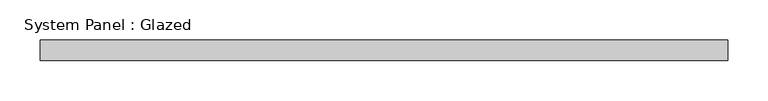
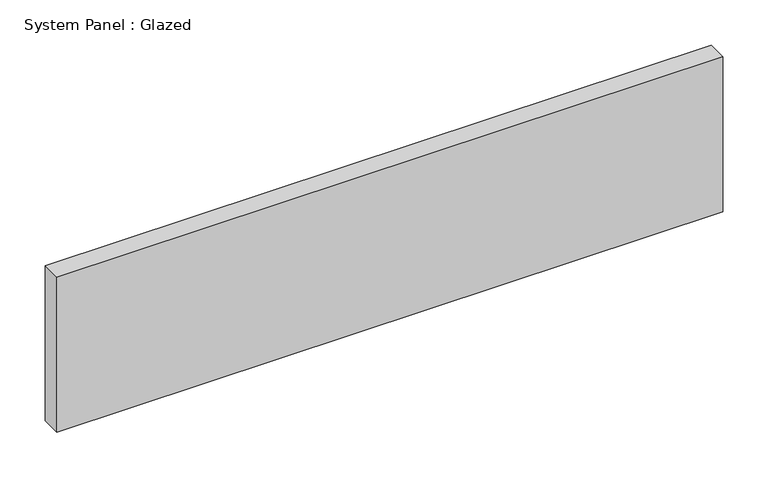
"""IFC4 building model written with IfcOpenShell, lengths in millimetres: plate geometry, System Panel : Glazed."""

from ifc_helpers import new_model, si_unit, origin, origin_with_axes, place, context, project, spatial, polyline, outline, extrude, source, transform, mapped, element, save


def system_panel_glazed_fbb6c980(model_context):
    return source(origin(), model_context, "Body", "SweptSolid", [
        extrude(outline(polyline([(425.45, 19.05), (-425.45, 19.05), (-425.45, 44.45), (425.45, 44.45), (425.45, 19.05)])), origin_with_axes(), (0.0, 0.0, 1.0), 209.55),
    ])


if __name__ == "__main__":
    model = new_model("IFC4")
    model_context = context("Model", 3, world=origin())
    ifc_project = project(units=[si_unit("LENGTHUNIT", "METRE", prefix="MILLI")], contexts=[model_context])
    site = spatial("IfcSite", under=ifc_project)
    building = spatial("IfcBuilding", under=site)
    placement = place(None, origin())
    system_panel_glazed_shape = system_panel_glazed_fbb6c980(model_context)
    element("IfcPlate", 1, ObjectType="System Panel : Glazed", at=placement, inside=building, context=model_context, shape_type="MappedRepresentation", body=[
        mapped(system_panel_glazed_shape, transform((0.0, 0.0, 0.0), x_axis=(1.0, 0.0, 0.0), y_axis=(0.0, 1.0, 0.0), z_axis=(0.0, 0.0, 1.0))),
    ])
    save(model, "model.ifc")

# Revit data of these elements
# Type "System Panel : Glazed"
#   Construction Type Id = "GSP4R"
#   Analytic Construction = "1/8 in Pilkington single glazing"
#   Visual Light Transmittance = 0.9
#   Solar Heat Gain Coefficient = 0.86
#   Heat Transfer Coefficient (U) = 1.18115 BTU/(h·ft²·°F)
#   Define Thermal Properties by = 1
# Element 1 (IfcPlate, "System Panel : Glazed")
#   Materials on its faces: "Glass"
# Materials
#   "Glass": class "Glass", colour RGB 0 128 192, transparency 0.75, Description = "Soda Lime Glass", Cost = 0
